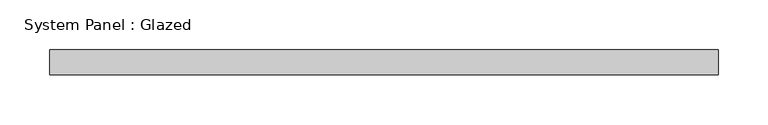
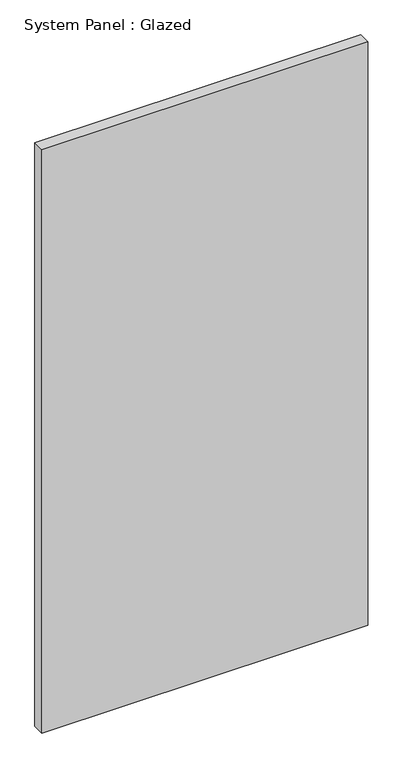
"""IFC4 building model written with IfcOpenShell, lengths in millimetres: plate geometry, System Panel : Glazed."""

from ifc_helpers import new_model, si_unit, origin, origin_with_axes, place, context, project, spatial, polyline, outline, extrude, source, transform, mapped, element, save


def system_panel_glazed_db295b58(model_context):
    return source(origin(), model_context, "Body", "SweptSolid", [
        extrude(outline(polyline([(337.2685902, 19.05), (-337.2685902, 19.05), (-337.2685902, 44.45), (337.2685902, 44.45), (337.2685902, 19.05)])), origin_with_axes(), (0.0, 0.0, 1.0), 1276.35),
    ])


if __name__ == "__main__":
    model = new_model("IFC4")
    model_context = context("Model", 3, world=origin())
    ifc_project = project(units=[si_unit("LENGTHUNIT", "METRE", prefix="MILLI")], contexts=[model_context])
    site = spatial("IfcSite", under=ifc_project)
    building = spatial("IfcBuilding", under=site)
    placement = place(None, origin())
    system_panel_glazed_shape = system_panel_glazed_db295b58(model_context)
    element("IfcPlate", 1, ObjectType="System Panel : Glazed", at=placement, inside=building, context=model_context, shape_type="MappedRepresentation", body=[
        mapped(system_panel_glazed_shape, transform((0.0, 0.0, 0.0), x_axis=(1.0, 0.0, 0.0), y_axis=(0.0, 1.0, 0.0), z_axis=(0.0, 0.0, 1.0))),
    ])
    save(model, "model.ifc")

# Revit data of these elements
# Type "System Panel : Glazed"
#   Construction Type Id = "GSP4R"
#   Analytic Construction = "1/8 in Pilkington single glazing"
#   Visual Light Transmittance = 0.9
#   Solar Heat Gain Coefficient = 0.86
#   Heat Transfer Coefficient (U) = 1.18115 BTU/(h·ft²·°F)
#   Define Thermal Properties by = 1
# Element 1 (IfcPlate, "System Panel : Glazed")
#   Materials on its faces: "Glass"
# Materials
#   "Glass": class "Glass", colour RGB 0 128 192, transparency 0.75, Description = "Soda Lime Glass", Cost = 0
